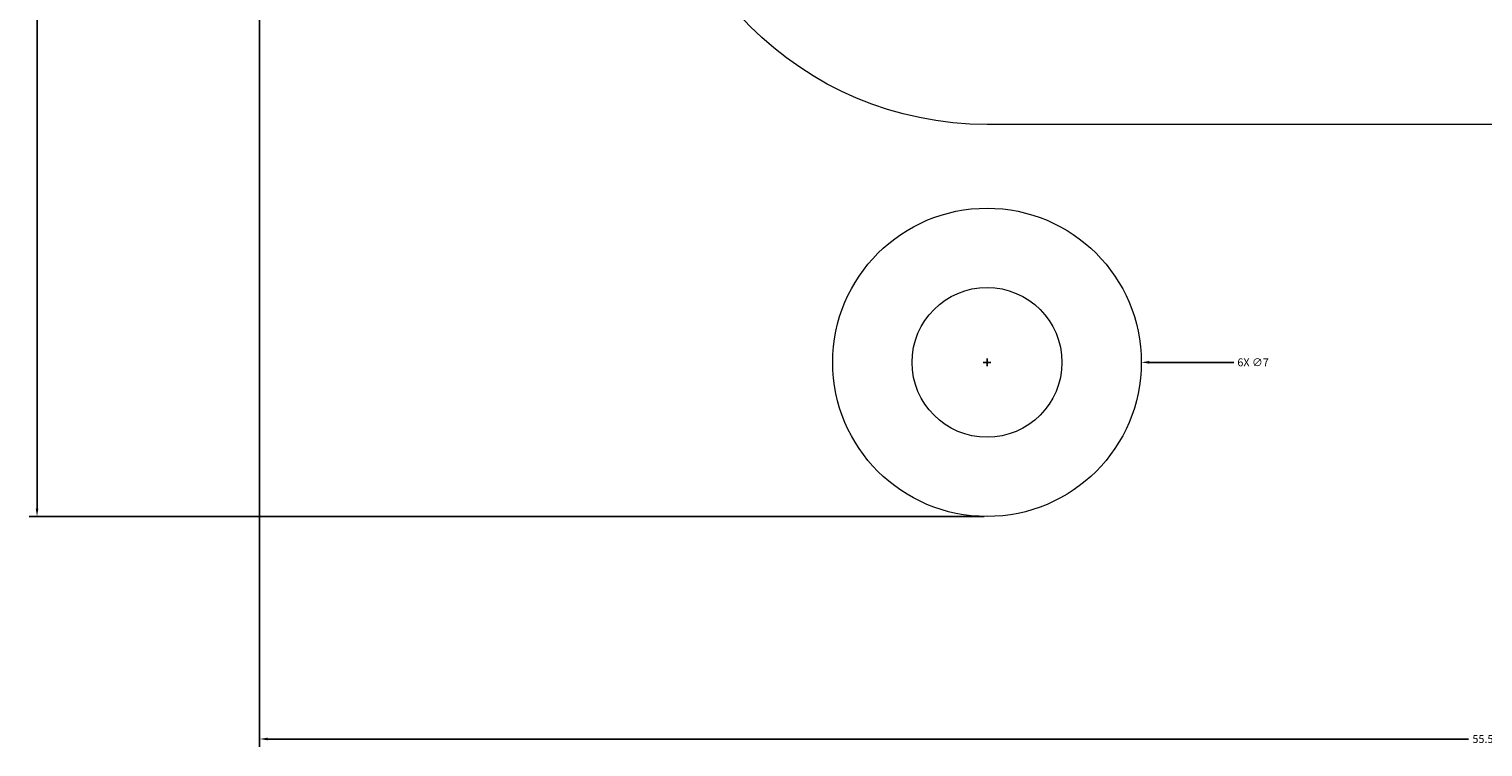
# Model space of a CAD drawing. Units: millimetres. Extents: x 3243.8 to 3309.8, y 1625.7 to 1669.2.
# Tile 1 of 3: x 3243.8 to 3276.8, y 1625.7 to 1642. Entities that reach past the tile are written whole.
import ezdxf

# ---------------------------------------------------------------- set-up
doc = ezdxf.new("R2010")
doc.units = ezdxf.units.MM
doc.layers.add('M-CONS', color=8, linetype='Continuous', lineweight=18)
doc.layers.add('M-DIMS', color=2, linetype='Continuous', lineweight=18)
doc.styles.get("Standard").update_dxf_attribs({"font": 'arial.ttf'})
doc.dimstyles.get("Standard").update_dxf_attribs({"dimtxt": 0.18, "dimasz": 0.18, "dimexe": 0.18, "dimexo": 0.0625, "dimgap": 0.09, "dimtad": 0, "dimtih": 1, "dimtoh": 1, "dimdec": 4, "dimzin": 0, "dimdsep": 46, "dimtxsty": 'Standard', "dimcen": 0.09, "dimadec": 0, "dimazin": 0, "dimtfac": 1, "dimtdec": 4, "dimtofl": 0, "dimtmove": 0, "dimatfit": 3, "dimfxl": 1, "dimtolj": 1, "dimtzin": 0, "dimarcsym": 0})

# ---------------------------------------------------------------- blocks, each defined once
blk = doc.blocks.new('CBORE-7-BORE-3.4')
for centre, radius in [((3.5, 3.5), 3.5), ((3.5, 3.5, -1), 1.7)]:
    blk.add_circle(centre, radius)
blk = doc.blocks.new('*D2')
at = {"layer": 'Defpoints', "color": 0, "transparency": 16777216}
for p in [(3249.045, 1647.47), (3304.545, 1647.47), (3304.545, 1625.92)]:
    blk.add_point(p, dxfattribs=at)
at = {"layer": 'M-DIMS', "color": 0, "lineweight": -2, "transparency": 16777216}
for p, q in [((3249.045, 1647.407), (3249.045, 1625.74)), ((3304.545, 1647.407), (3304.545, 1625.74)), ((3249.225, 1625.92), (3276.47, 1625.92)), ((3304.365, 1625.92), (3277.119, 1625.92))]:
    blk.add_line(p, q, dxfattribs=at)
at = {"layer": 'M-DIMS', "color": 0, "transparency": 16777216}
for points in [[(3249.225, 1625.95), (3249.225, 1625.89), (3249.045, 1625.92)], [(3304.365, 1625.95), (3304.365, 1625.89), (3304.545, 1625.92)]]:
    blk.add_solid(points, dxfattribs=at)
at = {"layer": 'M-DIMS', "color": 0, "transparency": 16777216, "insert": (3276.795, 1625.92), "char_height": 0.18, "attachment_point": 5}
blk.add_mtext('\\A1;55.5', dxfattribs=at)
blk = doc.blocks.new('*D3')
at = {"layer": 'Defpoints', "color": 0, "transparency": 16777216}
for p in [(3243.995, 1663.97), (3265.545, 1663.97), (3265.545, 1630.97)]:
    blk.add_point(p, dxfattribs=at)
at = {"layer": 'M-DIMS', "color": 0, "lineweight": -2, "transparency": 16777216}
for p, q in [((3265.482, 1663.97), (3243.815, 1663.97)), ((3243.995, 1663.79), (3243.995, 1647.652)), ((3243.995, 1631.15), (3243.995, 1647.288)), ((3265.482, 1630.97), (3243.815, 1630.97))]:
    blk.add_line(p, q, dxfattribs=at)
at = {"layer": 'M-DIMS', "color": 0, "transparency": 16777216}
for points in [[(3243.965, 1663.79), (3244.025, 1663.79), (3243.995, 1663.97)], [(3243.965, 1631.15), (3244.025, 1631.15), (3243.995, 1630.97)]]:
    blk.add_solid(points, dxfattribs=at)
at = {"layer": 'M-DIMS', "color": 0, "transparency": 16777216, "insert": (3243.995, 1647.47), "char_height": 0.18, "attachment_point": 5}
blk.add_mtext('\\A1;33', dxfattribs=at)
blk = doc.blocks.new('*D9')
at = {"layer": 'Defpoints', "color": 0, "transparency": 16777216}
for p in [(3262.045, 1634.47), (3269.045, 1634.47)]:
    blk.add_point(p, dxfattribs=at)
at = {"layer": 'M-DIMS', "color": 0, "lineweight": -2, "transparency": 16777216}
for p, q in [((3265.545, 1634.38), (3265.545, 1634.56)), ((3265.455, 1634.47), (3265.635, 1634.47)), ((3271.145, 1634.47), (3269.225, 1634.47))]:
    blk.add_line(p, q, dxfattribs=at)
at = {"layer": 'M-DIMS', "color": 0, "transparency": 16777216}
blk.add_solid([(3269.225, 1634.5), (3269.225, 1634.44), (3269.045, 1634.47)], dxfattribs=at)
at = {"layer": 'M-DIMS', "color": 0, "transparency": 16777216, "insert": (3271.581, 1634.47), "char_height": 0.18, "attachment_point": 5}
blk.add_mtext('\\A1;6X ∅7', dxfattribs=at)

msp = doc.modelspace()

# ---------------------------------------------------------------- linework, layer by layer
at = {"layer": 'M-CONS'}
msp.add_lwpolyline([(3265.545, 1655.07), (3288.045, 1655.07, -1), (3288.045, 1639.87), (3265.545, 1639.87, -1)], format="xyb", close=True, dxfattribs=at)
for centre, radius in [((3265.545, 1634.47), 3.5), ((3265.545, 1634.47, -1), 1.7)]:
    msp.add_circle(centre, radius, dxfattribs=at)

# ---------------------------------------------------------------- block references
msp.add_blockref('CBORE-7-BORE-3.4', (3262.045, 1630.97), dxfattribs=at)

# ---------------------------------------------------------------- dimensions: what is measured, and where the dimension line sits
at = {"layer": 'M-DIMS'}
dim = msp.add_linear_dim(base=(3243.995, 1663.97), p1=(3265.545, 1630.97), p2=(3265.545, 1663.97), angle=90, dimstyle='Standard', override={"dimdec": 0, "dimlfac": 1, "dimrnd": 0, "dimzin": 0, "dimdsep": 46, "dimlunit": 2}, dxfattribs=at)
dim.commit()
dim.dimension.update_dxf_attribs({"geometry": '*D3', "text_midpoint": (3243.995, 1647.47)})
dim = msp.add_linear_dim(base=(3304.545, 1625.92), p1=(3249.045, 1647.47), p2=(3304.545, 1647.47), dimstyle='Standard', override={"dimdec": 1, "dimlfac": 1, "dimrnd": 0, "dimzin": 0, "dimdsep": 46, "dimlunit": 2}, dxfattribs=at)
dim.commit()
dim.dimension.update_dxf_attribs({"geometry": '*D2', "text_midpoint": (3276.795, 1625.92)})
dim = msp.add_diameter_dim_2p(p1=(3262.045, 1634.47), p2=(3269.045, 1634.47), text='6X <>', dimstyle='Standard', override={"dimdec": 0, "dimlfac": 1, "dimrnd": 0, "dimzin": 0, "dimdsep": 46, "dimlunit": 2}, dxfattribs=at)
dim.commit()
dim.dimension.update_dxf_attribs({"geometry": '*D9', "text_midpoint": (3271.145, 1634.47), "dimtype": 163})

doc.saveas('drawing.dxf')
